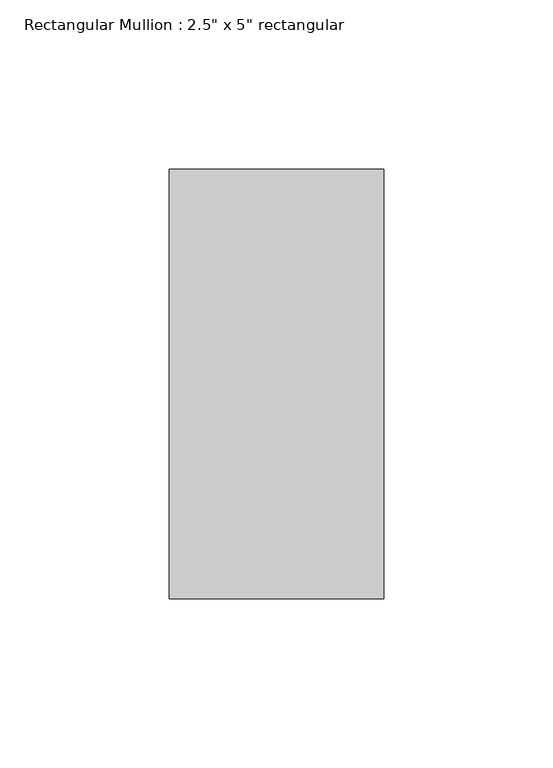
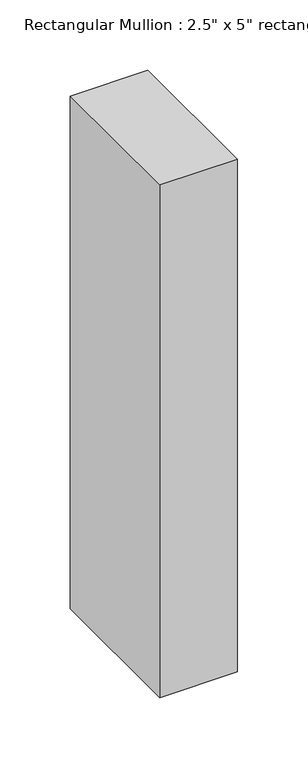
"""IFC4 building model written with IfcOpenShell, lengths in millimetres: member geometry."""

from ifc_helpers import new_model, si_unit, frame, origin, place, context, project, spatial, polyline, outline, extrude, source, transform, mapped, element, save


def member_663db4d7(model_context):
    return source(origin(), model_context, "Body", "SweptSolid", [
        extrude(outline(polyline([(31.75, 63.5), (31.75, -63.5), (-31.75, -63.5), (-31.75, 63.5), (31.75, 63.5)])), frame((0.0, 0.0, -444.7313568), z_axis=(0.0, 0.0, 1.0), x_axis=(1.0, 0.0, 0.0)), (0.0, 0.0, 1.0), 444.7313568),
    ])


if __name__ == "__main__":
    model = new_model("IFC4")
    model_context = context("Model", 3, world=origin())
    ifc_project = project(units=[si_unit("LENGTHUNIT", "METRE", prefix="MILLI")], contexts=[model_context])
    site = spatial("IfcSite", under=ifc_project)
    building = spatial("IfcBuilding", under=site)
    placement = place(None, origin())
    member_shape = member_663db4d7(model_context)
    element("IfcMember", 1, ObjectType="Rectangular Mullion : 2.5\" x 5\" rectangular", at=placement, inside=building, context=model_context, shape_type="MappedRepresentation", body=[
        mapped(member_shape, transform((0.0, 0.0, 0.0), x_axis=(1.0, 0.0, 0.0), y_axis=(0.0, 1.0, 0.0), z_axis=(0.0, 0.0, 1.0))),
    ])
    save(model, "model.ifc")

# Revit data of these elements
# Type "Rectangular Mullion : 2.5\" x 5\" rectangular"
#   built-in parameter 1007304 = 0.416667 (stored number, unit not read)
#   built-in parameter 1007301 = 0.104167 (stored number, unit not read)
#   built-in parameter 1007300 = 0.104167 (stored number, unit not read)
# Element 1 (IfcMember, "Rectangular Mullion : 2.5\" x 5\" rectangular")
#   Materials on its faces: "Aluminum"
# Materials
#   "Aluminum": class "Metal", colour RGB 247 247 247, transparency 0, Description = "Aluminum 6061", Cost = 0
